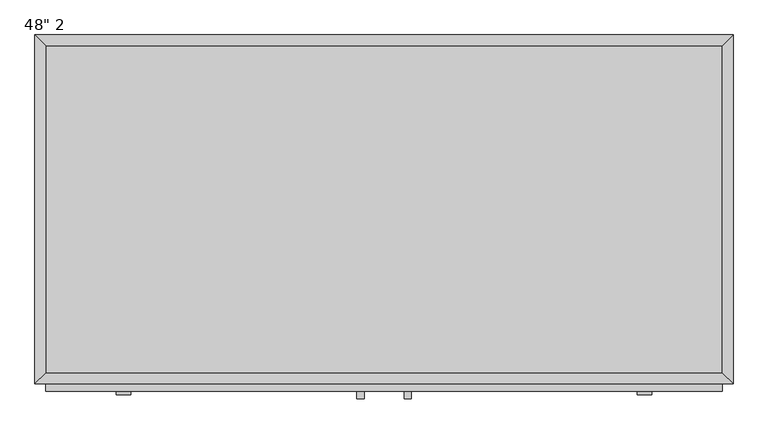
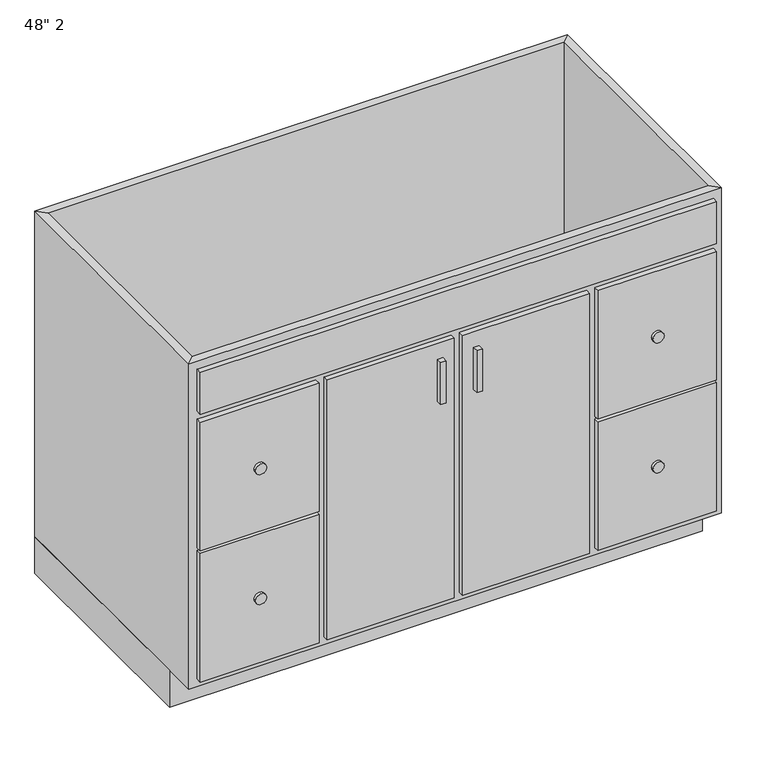
"""IFC4 building model written with IfcOpenShell, lengths in millimetres: furniture geometry."""

from ifc_helpers import new_model, si_unit, point, frame, frame_2d, origin, origin_with_axes, place, context, project, spatial, polyline, circle_curve, trimmed, segment, composite_curve, outline, extrude, faceted_brep, source, transform, mapped, element, save


def furniture_3428e43d(model_context):
    return source(origin(), model_context, "Body", "SolidModel", [
        extrude(outline(polyline([(700.44496, 0.0), (700.44496, -533.4), (-518.75504, -533.4), (-518.75504, 0.0), (700.44496, 0.0)])), origin_with_axes(), (0.0, 0.0, 1.0), 88.9),
        faceted_brep([(681.39496, -590.55, 876.3), (681.39496, -590.55, 88.9), (-499.70504, -590.55, 88.9), (-499.70504, -590.55, 876.3), (700.44496, -609.6, 876.3), (-518.75504, -609.6, 876.3), (700.44496, -609.6, 88.9), (-518.75504, -609.6, 88.9), (-499.70504, -19.05, 88.9), (-499.70504, -19.05, 876.3), (-518.75504, 0.0, 876.3), (-518.75504, 0.0, 88.9), (681.39496, -19.05, 88.9), (681.39496, -19.05, 876.3), (700.44496, 0.0, 876.3), (700.44496, 0.0, 88.9)], [[[0, 1, 2, 3]], [[4, 0, 3, 5]], [[6, 4, 5, 7]], [[1, 6, 7, 2]], [[3, 2, 8, 9]], [[5, 3, 9, 10]], [[7, 5, 10, 11]], [[2, 7, 11, 8]], [[9, 8, 12, 13]], [[10, 9, 13, 14]], [[11, 10, 14, 15]], [[8, 11, 15, 12]], [[13, 12, 1, 0]], [[14, 13, 0, 4]], [[15, 14, 4, 6]], [[12, 15, 6, 1]]]),
        extrude(outline(polyline([(681.39496, -19.05), (681.39496, -590.55), (-499.70504, -590.55), (-499.70504, -19.05), (681.39496, -19.05)])), frame((0.0, 0.0, 88.9), z_axis=(0.0, 0.0, 1.0), x_axis=(1.0, 0.0, 0.0)), (0.0, 0.0, 1.0), 19.05),
        extrude(outline(composite_curve([segment(trimmed(circle_curve(frame_2d((265.1125, 545.66371)), 12.7), [point((265.1125, 532.96371))], [point((265.1125, 558.36371))], False, "CARTESIAN"), True, "CONTINUOUS"), segment(trimmed(circle_curve(frame_2d((265.1125, 545.66371)), 12.7), [point((265.1125, 558.36371))], [point((265.1125, 532.96371))], False, "CARTESIAN"), True, "CONTINUOUS")], self_intersect=False)), frame((0.0, -628.65, 0.0), z_axis=(0.0, 1.0, 0.0), x_axis=(0.0, 0.0, 1.0)), (0.0, 0.0, 1.0), 6.35),
        extrude(outline(composite_curve([segment(trimmed(circle_curve(frame_2d((579.4375, 545.66371)), 12.7), [point((579.4375, 532.96371))], [point((579.4375, 558.36371))], False, "CARTESIAN"), True, "CONTINUOUS"), segment(trimmed(circle_curve(frame_2d((579.4375, 545.66371)), 12.7), [point((579.4375, 558.36371))], [point((579.4375, 532.96371))], False, "CARTESIAN"), True, "CONTINUOUS")], self_intersect=False)), frame((0.0, -628.65, 0.0), z_axis=(0.0, 1.0, 0.0), x_axis=(0.0, 0.0, 1.0)), (0.0, 0.0, 1.0), 6.35),
        extrude(outline(composite_curve([segment(trimmed(circle_curve(frame_2d((579.4375, -363.97379)), 12.7), [point((579.4375, -376.67379))], [point((579.4375, -351.27379))], False, "CARTESIAN"), True, "CONTINUOUS"), segment(trimmed(circle_curve(frame_2d((579.4375, -363.97379)), 12.7), [point((579.4375, -351.27379))], [point((579.4375, -376.67379))], False, "CARTESIAN"), True, "CONTINUOUS")], self_intersect=False)), frame((0.0, -628.65, 0.0), z_axis=(0.0, 1.0, 0.0), x_axis=(0.0, 0.0, 1.0)), (0.0, 0.0, 1.0), 6.35),
        extrude(outline(composite_curve([segment(trimmed(circle_curve(frame_2d((265.1125, -363.97379)), 12.7), [point((265.1125, -376.67379))], [point((265.1125, -351.27379))], False, "CARTESIAN"), True, "CONTINUOUS"), segment(trimmed(circle_curve(frame_2d((265.1125, -363.97379)), 12.7), [point((265.1125, -351.27379))], [point((265.1125, -376.67379))], False, "CARTESIAN"), True, "CONTINUOUS")], self_intersect=False)), frame((0.0, -628.65, 0.0), z_axis=(0.0, 1.0, 0.0), x_axis=(0.0, 0.0, 1.0)), (0.0, 0.0, 1.0), 6.35),
        extrude(outline(polyline([(55.91996, -635.0), (43.21996, -635.0), (43.21996, -622.3), (55.91996, -622.3), (55.91996, -635.0)])), frame((0.0, 0.0, 596.9), z_axis=(0.0, 0.0, 1.0), x_axis=(1.0, 0.0, 0.0)), (0.0, 0.0, 1.0), 101.6),
        extrude(outline(polyline([(138.46996, -635.0), (125.76996, -635.0), (125.76996, -622.3), (138.46996, -622.3), (138.46996, -635.0)])), frame((0.0, 0.0, 596.9), z_axis=(0.0, 0.0, 1.0), x_axis=(1.0, 0.0, 0.0)), (0.0, 0.0, 1.0), 101.6),
        extrude(outline(polyline([(681.39496, -622.3), (-499.70504, -622.3), (-499.70504, -609.6), (681.39496, -609.6), (681.39496, -622.3)])), frame((0.0, 0.0, 755.65), z_axis=(0.0, 0.0, 1.0), x_axis=(1.0, 0.0, 0.0)), (0.0, 0.0, 1.0), 101.6),
        extrude(outline(polyline([(681.39496, -622.3), (409.93246, -622.3), (409.93246, -609.6), (681.39496, -609.6), (681.39496, -622.3)])), frame((0.0, 0.0, 425.45), z_axis=(0.0, 0.0, 1.0), x_axis=(1.0, 0.0, 0.0)), (0.0, 0.0, 1.0), 311.15),
        extrude(outline(polyline([(681.39496, -622.3), (409.93246, -622.3), (409.93246, -609.6), (681.39496, -609.6), (681.39496, -622.3)])), frame((0.0, 0.0, 107.95), z_axis=(0.0, 0.0, 1.0), x_axis=(1.0, 0.0, 0.0)), (0.0, 0.0, 1.0), 311.15),
        extrude(outline(polyline([(-228.24254, -622.3), (-499.70504, -622.3), (-499.70504, -609.6), (-228.24254, -609.6), (-228.24254, -622.3)])), frame((0.0, 0.0, 425.45), z_axis=(0.0, 0.0, 1.0), x_axis=(1.0, 0.0, 0.0)), (0.0, 0.0, 1.0), 311.15),
        extrude(outline(polyline([(-228.24254, -622.3), (-499.70504, -622.3), (-499.70504, -609.6), (-228.24254, -609.6), (-228.24254, -622.3)])), frame((0.0, 0.0, 107.95), z_axis=(0.0, 0.0, 1.0), x_axis=(1.0, 0.0, 0.0)), (0.0, 0.0, 1.0), 311.15),
        extrude(outline(polyline([(81.31996, -622.3), (-209.19254, -622.3), (-209.19254, -609.6), (81.31996, -609.6), (81.31996, -622.3)])), frame((0.0, 0.0, 107.95), z_axis=(0.0, 0.0, 1.0), x_axis=(1.0, 0.0, 0.0)), (0.0, 0.0, 1.0), 628.65),
        extrude(outline(polyline([(390.88246, -622.3), (100.36996, -622.3), (100.36996, -609.6), (390.88246, -609.6), (390.88246, -622.3)])), frame((0.0, 0.0, 107.95), z_axis=(0.0, 0.0, 1.0), x_axis=(1.0, 0.0, 0.0)), (0.0, 0.0, 1.0), 628.65),
    ])


if __name__ == "__main__":
    model = new_model("IFC4")
    model_context = context("Model", 3, world=origin())
    ifc_project = project(units=[si_unit("LENGTHUNIT", "METRE", prefix="MILLI")], contexts=[model_context])
    site = spatial("IfcSite", under=ifc_project)
    building = spatial("IfcBuilding", under=site)
    placement = place(None, origin())
    furniture_shape = furniture_3428e43d(model_context)
    element("IfcFurniture", 1, ObjectType="48\" 2", at=placement, inside=building, context=model_context, shape_type="MappedRepresentation", body=[
        mapped(furniture_shape, transform((0.0, 0.0, 0.0), x_axis=(1.0, 0.0, 0.0), y_axis=(0.0, 1.0, 0.0), z_axis=(0.0, 0.0, 1.0))),
    ])
    save(model, "model.ifc")

# Revit data of these elements
# Type "48\" 2"
#   Assembly Code = "C1030410"
#   Depth = 2' - 0"
#   Height = 2' - 10 1/2"
#   Toe Depth = 0' - 3"
#   Toe Height = 0' - 3 1/2"
#   Width = 4' - 0"
#   Cabinet Material = none
#   Door/Drawer Material = none
#   Handle Material = Cabinets - Handles
#   Default Elevation = 0
# Element 1 (IfcFurniture, "48\" 2")
#   Materials on its faces: "Cabinets", "Cabinets - Handles"
# Materials
#   "Cabinets - Handles": class "Metal", colour RGB 57 57 57, transparency 0
#   "Cabinets": colour RGB 249 249 249, transparency 0
